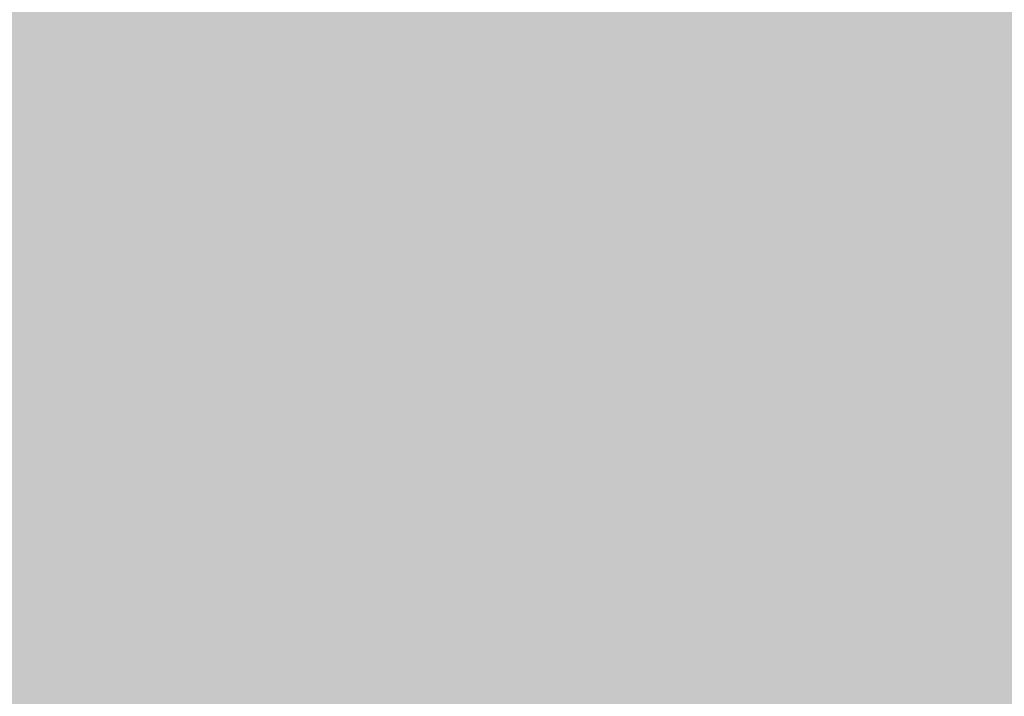
# Model space of a CAD drawing. Units: millimetres. Extents: x 0 to 2267, y 0 to 1823.
# Tile 75 of 256: x 1596.855 to 1600.369, y 1228.528 to 1230.942. Entities that reach past the tile are written whole.
import ezdxf

# ---------------------------------------------------------------- set-up
doc = ezdxf.new("R2010")
doc.units = ezdxf.units.MM
doc.header["$MEASUREMENT"] = 0
doc.layers.add('M-HATC', color=252, linetype='Continuous', lineweight=18)

msp = doc.modelspace()

# ---------------------------------------------------------------- hatches: boundary and pattern name
at = {"layer": 'M-HATC'}
h = msp.add_hatch(color=256, dxfattribs=at)
h.dxf.hatch_style = 1
h.paths.add_polyline_path([(2055.771, 1603.062), (1381.0868, 1603.062), (1381.0868, 1598.062), (2055.771, 1598.062)])
h.paths.add_polyline_path([(2055.771, 1598.062), (1381.0868, 1598.062), (1381.0868, 1593.062), (2055.771, 1593.062)])
h.paths.add_polyline_path([(2051.3074, 1536.7609), (1385.5504, 1536.7609), (1385.5504, 1526.7609), (1387.5504, 1526.7609), (1388.5366, 1525.0528), (1385.3319, 1521.2335), (1385.3319, 1521.2226), (2050.2542, 1522.7491), (2048.3212, 1525.0528), (2049.3074, 1526.7609), (2051.3074, 1526.7609)])
edge = h.paths.add_edge_path()
edge.add_arc((1847.5345, 1379.1492), 135, 222.603061, 222.890851, ccw=False)
edge.add_line((1748.1663, 1287.7656), (1683.0921, 1287.7656))
edge.add_arc((1583.7239, 1379.1492), 135, 317.109149, 317.396939, ccw=False)
edge.add_arc((1678.9686, 1290.6707), 5, 222.8909, 317.1091, ccw=False)
edge.add_arc((1774.2133, 1379.1492), 135, 222.603061, 222.890851, ccw=False)
edge.add_line((1674.8451, 1287.7656), (1609.7709, 1287.7656))
edge.add_arc((1510.4027, 1379.1492), 135, 317.109149, 317.396939, ccw=False)
edge.add_arc((1605.6474, 1290.6707), 5, 222.8909, 317.1091, ccw=False)
edge.add_arc((1700.8921, 1379.1492), 135, 222.603061, 222.890851, ccw=False)
edge.add_line((1601.5239, 1287.7656), (1536.4497, 1287.7656))
edge.add_arc((1437.0815, 1379.1492), 135, 317.109149, 317.396939, ccw=False)
edge.add_arc((1532.3262, 1290.6707), 5, 222.8909, 317.1091, ccw=False)
edge.add_arc((1627.5709, 1379.1492), 135, 222.603061, 222.890851, ccw=False)
edge.add_line((1528.2027, 1287.7656), (1505.9289, 1287.7656))
edge.add_spline(control_points=[(1505.9289, 1287.7656), (1504.2622, 1287.7656), (1504.2622, 1282.7656), (1505.9289, 1282.7656)], knot_values=[0, 0, 0, 0, 5, 5, 5, 5], degree=3, periodic=0)
edge.add_line((1505.9289, 1282.7656), (1930.9289, 1282.7656))
edge.add_spline(control_points=[(1930.9289, 1282.7656), (1932.5956, 1282.7656), (1932.5956, 1287.7656), (1930.9289, 1287.7656)], knot_values=[0, 0, 0, 0, 5, 5, 5, 5], degree=3, periodic=0)
edge.add_line((1930.9289, 1287.7656), (1903.0557, 1287.7656))
edge.add_arc((1803.6875, 1379.1492), 135, 317.109149, 317.396939, ccw=False)
edge.add_arc((1898.9322, 1290.6707), 5, 222.8909, 317.1091, ccw=False)
edge.add_arc((1994.1769, 1379.1492), 135, 222.603061, 222.890851, ccw=False)
edge.add_line((1894.8087, 1287.7656), (1829.7345, 1287.7656))
edge.add_arc((1730.3663, 1379.1492), 135, 317.109149, 317.396939, ccw=False)
edge.add_arc((1825.611, 1290.6707), 5, 222.8909, 317.1091, ccw=False)
edge.add_arc((1920.8557, 1379.1492), 135, 222.603061, 222.890851, ccw=False)
edge.add_line((1821.4875, 1287.7656), (1756.4133, 1287.7656))
edge.add_arc((1657.0451, 1379.1492), 135, 317.109149, 317.396939, ccw=False)
edge.add_arc((1752.2898, 1290.6707), 5, 222.8909, 317.1091, ccw=False)
edge = h.paths.add_edge_path()
edge.add_spline(control_points=[(1843.4289, 1227.2475), (1845.0956, 1227.2475), (1845.0956, 1232.2475), (1843.4289, 1232.2475)], knot_values=[0, 0, 0, 0, 5, 5, 5, 5], degree=3, periodic=0)
edge.add_line((1843.4289, 1232.2475), (1593.4289, 1232.2475))
edge.add_spline(control_points=[(1593.4289, 1232.2475), (1591.7622, 1232.2475), (1591.7622, 1227.2475), (1593.4289, 1227.2475)], knot_values=[0, 0, 0, 0, 5, 5, 5, 5], degree=3, periodic=0)
edge.add_line((1593.4289, 1227.2475), (1843.4289, 1227.2475))
h.paths.add_polyline_path([(1905.9289, 1127.4171), (1530.9289, 1127.4171, 0.414214), (1520.9289, 1117.4171), (1530.9289, 1117.4171), (1915.9289, 1117.4171, 0.414214)])
edge = h.paths.add_edge_path()
edge.add_arc((1397.0858, 1498.4078), 12.7299, 90.78215, 190.87871, ccw=False)
edge.add_line((1396.912, 1511.1365), (1428.0097, 1511.3488))
edge.add_line((1428.0097, 1511.3488), (1433.0097, 1511.3488))
edge.add_line((1433.0097, 1511.3488), (1434.439, 1511.3488))
edge.add_arc((1419.474, 1498.0804), 20, 41.561, 74.08211)
edge.add_line((1424.9592, 1517.3135), (1399.9351, 1517.2561))
edge.add_spline(control_points=[(1399.9307, 1517.2561), (1399.884, 1517.2131), (1399.8328, 1517.1689), (1399.7774, 1517.1236)], knot_values=[11.567499, 11.567499, 11.567499, 11.567499, 11.814249, 11.814249, 11.814249, 11.814249], degree=3, periodic=0)
edge.add_spline(control_points=[(1399.6328, 1517.0099), (1399.5831, 1516.9721), (1399.5307, 1516.9338), (1399.4759, 1516.8947)], knot_values=[11.167718, 11.167718, 11.167718, 11.167718, 11.365188, 11.365188, 11.365188, 11.365188], degree=3, periodic=0)
edge.add_spline(control_points=[(1399.3398, 1516.8001), (1399.1514, 1516.6719), (1398.9384, 1516.5377), (1398.704, 1516.3994)], knot_values=[10.376405, 10.376405, 10.376405, 10.376405, 11.00994, 11.00994, 11.00994, 11.00994], degree=3, periodic=0)
edge.add_spline(control_points=[(1398.6572, 1516.3719), (1398.5789, 1516.326), (1398.4983, 1516.2797), (1398.4155, 1516.2331)], knot_values=[10.125175, 10.125175, 10.125175, 10.125175, 10.334406, 10.334406, 10.334406, 10.334406], degree=3, periodic=0)
edge.add_spline(control_points=[(1398.2642, 1516.1487), (1398.196, 1516.1111), (1398.1263, 1516.0732), (1398.0555, 1516.0351)], knot_values=[9.832246, 9.832246, 9.832246, 9.832246, 9.999658, 9.999658, 9.999658, 9.999658], degree=3, periodic=0)
edge.add_spline(control_points=[(1397.9987, 1516.0048), (1397.7312, 1515.8621), (1397.446, 1515.7171), (1397.1466, 1515.5714)], knot_values=[9.161808, 9.161808, 9.161808, 9.161808, 9.787769, 9.787769, 9.787769, 9.787769], degree=3, periodic=0)
edge.add_spline(control_points=[(1397.1466, 1515.5714), (1396.8418, 1515.423), (1396.5222, 1515.274), (1396.1914, 1515.1262)], knot_values=[8.524455, 8.524455, 8.524455, 8.524455, 9.161808, 9.161808, 9.161808, 9.161808], degree=3, periodic=0)
edge.add_spline(control_points=[(1396.0777, 1515.0756), (1395.9854, 1515.0348), (1395.8922, 1514.994), (1395.7983, 1514.9534)], knot_values=[8.275193, 8.275193, 8.275193, 8.275193, 8.451726, 8.451726, 8.451726, 8.451726], degree=3, periodic=0)
edge.add_spline(control_points=[(1395.6018, 1514.8691), (1395.4997, 1514.8257), (1395.3968, 1514.7824), (1395.2932, 1514.7394)], knot_values=[7.962917, 7.962917, 7.962917, 7.962917, 8.152764, 8.152764, 8.152764, 8.152764], degree=3, periodic=0)
edge.add_spline(control_points=[(1395.2116, 1514.7057), (1394.8278, 1514.5475), (1394.4345, 1514.3929), (1394.0364, 1514.2442)], knot_values=[7.21254, 7.21254, 7.21254, 7.21254, 7.913148, 7.913148, 7.913148, 7.913148], degree=3, periodic=0)
edge.add_spline(control_points=[(1394.0364, 1514.2442), (1393.7076, 1514.1214), (1393.3754, 1514.0027), (1393.0427, 1513.8895)], knot_values=[6.633733, 6.633733, 6.633733, 6.633733, 7.21254, 7.21254, 7.21254, 7.21254], degree=3, periodic=0)
edge.add_spline(control_points=[(1392.8214, 1513.815), (1392.7198, 1513.7812), (1392.6181, 1513.7479), (1392.5166, 1513.7152)], knot_values=[6.328796, 6.328796, 6.328796, 6.328796, 6.505493, 6.505493, 6.505493, 6.505493], degree=3, periodic=0)
edge.add_spline(control_points=[(1392.5166, 1513.7152), (1392.3187, 1513.6515), (1392.1212, 1513.59), (1391.9244, 1513.531)], knot_values=[5.984605, 5.984605, 5.984605, 5.984605, 6.328796, 6.328796, 6.328796, 6.328796], degree=3, periodic=0)
edge.add_spline(control_points=[(1391.7915, 1513.4915), (1391.3122, 1513.3501), (1390.8384, 1513.2239), (1390.3784, 1513.1171)], knot_values=[5.066697, 5.066697, 5.066697, 5.066697, 5.907055, 5.907055, 5.907055, 5.907055], degree=3, periodic=0)
edge.add_spline(control_points=[(1390.3784, 1513.1171), (1390.1797, 1513.071), (1389.9836, 1513.0284), (1389.7907, 1512.9899)], knot_values=[4.70367, 4.70367, 4.70367, 4.70367, 5.066695, 5.066695, 5.066695, 5.066695], degree=3, periodic=0)
edge.add_spline(control_points=[(1389.422, 1512.9204), (1389.2459, 1512.8892), (1389.0729, 1512.8617), (1388.9036, 1512.8381)], knot_values=[4.130571, 4.130571, 4.130571, 4.130571, 4.469816, 4.469816, 4.469816, 4.469816], degree=3, periodic=0)
edge.add_spline(control_points=[(1388.9036, 1512.8381), (1388.591, 1512.7946), (1388.2911, 1512.7644), (1388.0071, 1512.7494)], knot_values=[3.504031, 3.504031, 3.504031, 3.504031, 4.130571, 4.130571, 4.130571, 4.130571], degree=3, periodic=0)
edge.add_spline(control_points=[(1387.9356, 1512.7459), (1387.8538, 1512.7423), (1387.7733, 1512.74), (1387.6944, 1512.739)], knot_values=[3.268866, 3.268866, 3.268866, 3.268866, 3.451164, 3.451164, 3.451164, 3.451164], degree=3, periodic=0)
edge.add_spline(control_points=[(1387.3351, 1512.7443), (1387.2076, 1512.7499), (1387.0847, 1512.7597), (1386.967, 1512.7739)], knot_values=[2.670686, 2.670686, 2.670686, 2.670686, 2.984, 2.984, 2.984, 2.984], degree=3, periodic=0)
edge.add_spline(control_points=[(1386.8327, 1512.7922), (1386.8209, 1512.7941), (1386.8092, 1512.7959), (1386.7975, 1512.7979)], knot_values=[2.516981, 2.516981, 2.516981, 2.516981, 2.549528, 2.549528, 2.549528, 2.549528], degree=3, periodic=0)
edge.add_spline(control_points=[(1386.4526, 1512.8735), (1386.4257, 1512.881), (1386.3993, 1512.889), (1386.3733, 1512.8972)], knot_values=[2.095869, 2.095869, 2.095869, 2.095869, 2.17941, 2.17941, 2.17941, 2.17941], degree=3, periodic=0)
edge.add_spline(control_points=[(1386.0691, 1513.0189), (1386.0634, 1513.0217), (1386.0577, 1513.0246), (1386.052, 1513.0275)], knot_values=[1.72453, 1.72453, 1.72453, 1.72453, 1.745933, 1.745933, 1.745933, 1.745933], degree=3, periodic=0)
edge.add_arc((1399.474, 1498.0804), 20, 131.82432, 180)
edge.add_arc((1630.3336, 1505.5484), 250.9708, 181.705176, 236.427975)
edge.add_arc((1605.3399, 1483.3044), 218.7822, 238.660829, 243.34961)
edge.add_arc((1647.0911, 1510.3592), 262.8986, 183.129836, 237.853442, ccw=False)
h.paths.add_polyline_path([(1406.5369, 1391.9644, 0.149382), (1491.5506, 1296.4418, -0.129517)], flags=17)
edge = h.paths.add_edge_path()
edge.add_arc((2037.3838, 1498.0804), 20, 0, 48.26587)
edge.add_spline(control_points=[(2050.6973, 1513.0052), (2050.6512, 1512.9847), (2050.6034, 1512.9655), (2050.5539, 1512.9477)], knot_values=[1.835652, 1.835652, 1.835652, 1.835652, 2.000781, 2.000781, 2.000781, 2.000781], degree=3, periodic=0)
edge.add_spline(control_points=[(2050.4616, 1512.9166), (2050.479, 1512.9221), (2050.4963, 1512.9277), (2050.5133, 1512.9335)], knot_values=[2.045477, 2.045477, 2.045477, 2.045477, 2.101389, 2.101389, 2.101389, 2.101389], degree=3, periodic=0)
edge.add_spline(control_points=[(2050.129, 1512.8342), (2050.1984, 1512.8473), (2050.2657, 1512.8623), (2050.3308, 1512.8792)], knot_values=[2.237629, 2.237629, 2.237629, 2.237629, 2.435841, 2.435841, 2.435841, 2.435841], degree=3, periodic=0)
edge.add_spline(control_points=[(2050.0946, 1512.8278), (2050.1061, 1512.8299), (2050.1176, 1512.832), (2050.129, 1512.8342)], knot_values=[2.435841, 2.435841, 2.435841, 2.435841, 2.468321, 2.468321, 2.468321, 2.468321], degree=3, periodic=0)
edge.add_spline(control_points=[(2049.7843, 1512.7851), (2049.8552, 1512.7922), (2049.9243, 1512.8008), (2049.9917, 1512.8109)], knot_values=[2.563852, 2.563852, 2.563852, 2.563852, 2.748541, 2.748541, 2.748541, 2.748541], degree=3, periodic=0)
edge.add_spline(control_points=[(2049.4052, 1512.7617), (2049.5364, 1512.7653), (2049.6629, 1512.773), (2049.7843, 1512.7851)], knot_values=[2.748541, 2.748541, 2.748541, 2.748541, 3.064882, 3.064882, 3.064882, 3.064882], degree=3, periodic=0)
edge.add_spline(control_points=[(2049.1698, 1512.7597), (2049.2336, 1512.7591), (2049.2965, 1512.7594), (2049.3584, 1512.7606)], knot_values=[3.102309, 3.102309, 3.102309, 3.102309, 3.2503, 3.2503, 3.2503, 3.2503], degree=3, periodic=0)
edge.add_spline(control_points=[(2048.8573, 1512.7691), (2048.9638, 1512.7638), (2049.068, 1512.7606), (2049.1698, 1512.7597)], knot_values=[3.2503, 3.2503, 3.2503, 3.2503, 3.486069, 3.486069, 3.486069, 3.486069], degree=3, periodic=0)
edge.add_spline(control_points=[(2048.6924, 1512.7789), (2048.3729, 1512.8009), (2048.0345, 1512.8411), (2047.6817, 1512.897)], knot_values=[3.606429, 3.606429, 3.606429, 3.606429, 4.2989, 4.2989, 4.2989, 4.2989], degree=3, periodic=0)
edge.add_spline(control_points=[(2047.6817, 1512.897), (2047.5458, 1512.9185), (2047.4077, 1512.9424), (2047.2678, 1512.9685)], knot_values=[4.2989, 4.2989, 4.2989, 4.2989, 4.565769, 4.565769, 4.565769, 4.565769], degree=3, periodic=0)
edge.add_spline(control_points=[(2047.2678, 1512.9685), (2047.1449, 1512.9914), (2047.0207, 1513.016), (2046.8951, 1513.0422)], knot_values=[4.565769, 4.565769, 4.565769, 4.565769, 4.799971, 4.799971, 4.799971, 4.799971], degree=3, periodic=0)
edge.add_spline(control_points=[(2046.8951, 1513.0422), (2046.5286, 1513.1188), (2046.1513, 1513.209), (2045.7676, 1513.3107)], knot_values=[4.799971, 4.799971, 4.799971, 4.799971, 5.483718, 5.483718, 5.483718, 5.483718], degree=3, periodic=0)
edge.add_spline(control_points=[(2045.7676, 1513.3107), (2045.3724, 1513.4154), (2044.9704, 1513.5322), (2044.5662, 1513.6588)], knot_values=[5.483718, 5.483718, 5.483718, 5.483718, 6.187866, 6.187866, 6.187866, 6.187866], degree=3, periodic=0)
edge.add_spline(control_points=[(2044.5662, 1513.6588), (2044.4149, 1513.7061), (2044.2633, 1513.7549), (2044.1116, 1513.8048)], knot_values=[6.187866, 6.187866, 6.187866, 6.187866, 6.451551, 6.451551, 6.451551, 6.451551], degree=3, periodic=0)
edge.add_spline(control_points=[(2044.1116, 1513.8048), (2043.9967, 1513.8427), (2043.8817, 1513.8813), (2043.7668, 1513.9205)], knot_values=[6.451551, 6.451551, 6.451551, 6.451551, 6.651434, 6.651434, 6.651434, 6.651434], degree=3, periodic=0)
edge.add_spline(control_points=[(2043.7668, 1513.9205), (2043.3716, 1514.0554), (2042.9774, 1514.1979), (2042.5886, 1514.3458)], knot_values=[6.651434, 6.651434, 6.651434, 6.651434, 7.338879, 7.338879, 7.338879, 7.338879], degree=3, periodic=0)
edge.add_spline(control_points=[(2042.5886, 1514.3458), (2042.1643, 1514.5071), (2041.7465, 1514.6749), (2041.3409, 1514.846)], knot_values=[7.338879, 7.338879, 7.338879, 7.338879, 8.089209, 8.089209, 8.089209, 8.089209], degree=3, periodic=0)
edge.add_spline(control_points=[(2041.3409, 1514.846), (2041.1028, 1514.9465), (2040.869, 1515.0481), (2040.6405, 1515.1502)], knot_values=[8.089209, 8.089209, 8.089209, 8.089209, 8.529587, 8.529587, 8.529587, 8.529587], degree=3, periodic=0)
edge.add_spline(control_points=[(2040.51, 1515.2089), (2040.0824, 1515.4022), (2039.6747, 1515.5971), (2039.295, 1515.7894)], knot_values=[8.613818, 8.613818, 8.613818, 8.613818, 9.44571, 9.44571, 9.44571, 9.44571], degree=3, periodic=0)
edge.add_spline(control_points=[(2039.295, 1515.7894), (2039.0618, 1515.9075), (2038.8391, 1516.0246), (2038.6288, 1516.1398)], knot_values=[9.44571, 9.44571, 9.44571, 9.44571, 9.956404, 9.956404, 9.956404, 9.956404], degree=3, periodic=0)
edge.add_spline(control_points=[(2038.6288, 1516.1398), (2038.5187, 1516.2001), (2038.4121, 1516.2598), (2038.309, 1516.3189)], knot_values=[9.956404, 9.956404, 9.956404, 9.956404, 10.223542, 10.223542, 10.223542, 10.223542], degree=3, periodic=0)
edge.add_spline(control_points=[(2038.309, 1516.3189), (2038.2138, 1516.3735), (2038.1216, 1516.4276), (2038.0328, 1516.481)], knot_values=[10.223542, 10.223542, 10.223542, 10.223542, 10.47051, 10.47051, 10.47051, 10.47051], degree=3, periodic=0)
edge.add_spline(control_points=[(2038.0328, 1516.481), (2037.7855, 1516.6296), (2037.5639, 1516.773), (2037.3722, 1516.909)], knot_values=[10.47051, 10.47051, 10.47051, 10.47051, 11.15767, 11.15767, 11.15767, 11.15767], degree=3, periodic=0)
edge.add_spline(control_points=[(2037.3722, 1516.909), (2037.2789, 1516.9752), (2037.1927, 1517.0396), (2037.1142, 1517.102)], knot_values=[11.15767, 11.15767, 11.15767, 11.15767, 11.49227, 11.49227, 11.49227, 11.49227], degree=3, periodic=0)
edge.add_spline(control_points=[(2036.8564, 1517.3259), (2036.9148, 1517.2692), (2036.9814, 1517.2103), (2037.0557, 1517.1492)], knot_values=[11.577341, 11.577341, 11.577341, 11.577341, 11.91035, 11.91035, 11.91035, 11.91035], degree=3, periodic=0)
edge.add_spline(control_points=[(2036.8074, 1517.3748), (2036.823, 1517.3587), (2036.8393, 1517.3424), (2036.8564, 1517.3259)], knot_values=[11.91035, 11.91035, 11.91035, 11.91035, 12.007402, 12.007402, 12.007402, 12.007402], degree=3, periodic=0)
edge.add_spline(control_points=[(2036.7017, 1517.494), (2036.7104, 1517.483), (2036.7196, 1517.4719), (2036.7291, 1517.4606)], knot_values=[12.184155, 12.184155, 12.184155, 12.184155, 12.255409, 12.255409, 12.255409, 12.255409], degree=3, periodic=0)
edge.add_spline(control_points=[(2036.6159, 1517.6205), (2036.62, 1517.613), (2036.6243, 1517.6055), (2036.6289, 1517.5979)], knot_values=[12.487913, 12.487913, 12.487913, 12.487913, 12.541035, 12.541035, 12.541035, 12.541035], degree=3, periodic=0)
edge.add_spline(control_points=[(2036.5635, 1517.786), (2036.5637, 1517.7794), (2036.5642, 1517.7726), (2036.565, 1517.7658)], knot_values=[12.911761, 12.911761, 12.911761, 12.911761, 12.968286, 12.968286, 12.968286, 12.968286], degree=3, periodic=0)
edge.add_spline(control_points=[(2036.6166, 1517.9304), (2036.6125, 1517.9259), (2036.6086, 1517.9212), (2036.6049, 1517.9165)], knot_values=[13.382527, 13.382527, 13.382527, 13.382527, 13.433791, 13.433791, 13.433791, 13.433791], degree=3, periodic=0)
edge.add_spline(control_points=[(2036.749, 1518.017), (2036.7361, 1518.0116), (2036.7239, 1518.006), (2036.7124, 1518.0002)], knot_values=[13.726299, 13.726299, 13.726299, 13.726299, 13.809928, 13.809928, 13.809928, 13.809928], degree=3, periodic=0)
edge.add_spline(control_points=[(2036.8604, 1518.0528), (2036.8386, 1518.0474), (2036.8181, 1518.0416), (2036.7988, 1518.0353)], knot_values=[13.910887, 13.910887, 13.910887, 13.910887, 14.02153, 14.02153, 14.02153, 14.02153], degree=3, periodic=0)
edge.add_line((2036.9639, 1518.0804), (2032.3838, 1518.0804))
edge.add_line((2032.3838, 1518.0804), (2027.3838, 1518.0804))
edge.add_line((2027.3838, 1518.0804), (2022.3838, 1518.0804))
edge.add_line((2022.3838, 1518.0804), (2017.3838, 1518.0804))
edge.add_arc((2017.3838, 1498.0804), 20, 90, 138.439)
edge.add_line((2002.4188, 1511.3488), (2003.8481, 1511.3488))
edge.add_line((2003.8481, 1511.3488), (2008.8481, 1511.3488))
edge.add_line((2008.8481, 1511.3488), (2039.772, 1511.1377))
edge.add_arc((2039.772, 1498.4078), 12.7299, -10.87871, 90, ccw=False)
edge.add_arc((1789.7668, 1510.3592), 262.8986, 302.146558, 356.870164, ccw=False)
edge.add_arc((1831.5179, 1483.3044), 218.7822, 296.65039, 301.339171)
edge.add_arc((1806.5242, 1505.5484), 250.9708, 303.572025, 358.294824)
h.paths.add_polyline_path([(2030.321, 1391.9644, -0.129517), (1945.3072, 1296.4418, 0.149382)], flags=17)
edge = h.paths.add_edge_path()
edge.add_spline(control_points=[(2037.2464, 1518.0821), (2037.2898, 1518.081), (2037.3355, 1518.0804), (2037.3838, 1518.0804)], knot_values=[0.000012, 0.000012, 0.000012, 0.000012, 0.144754, 0.144754, 0.144754, 0.144754], degree=3, periodic=0)
edge.add_line((2037.3357, 1518.0804), (2037.0096, 1518.0804))
edge.add_spline(control_points=[(2037.0096, 1518.0804), (2036.9822, 1518.0768), (2036.956, 1518.0727), (2036.9312, 1518.0681)], knot_values=[14.13465, 14.13465, 14.13465, 14.13465, 14.247197, 14.247197, 14.247197, 14.247197], degree=3, periodic=0)
edge.add_spline(control_points=[(2036.9312, 1518.0681), (2036.9276, 1518.0674), (2036.9241, 1518.0667), (2036.9205, 1518.0661)], knot_values=[14.118315, 14.118315, 14.118315, 14.118315, 14.13465, 14.13465, 14.13465, 14.13465], degree=3, periodic=0)
edge.add_spline(control_points=[(2036.9205, 1518.0661), (2036.9118, 1518.0644), (2036.9032, 1518.0626), (2036.8948, 1518.0608)], knot_values=[14.078086, 14.078086, 14.078086, 14.078086, 14.118315, 14.118315, 14.118315, 14.118315], degree=3, periodic=0)
edge.add_spline(control_points=[(2036.8948, 1518.0608), (2036.883, 1518.0583), (2036.8716, 1518.0556), (2036.8604, 1518.0528)], knot_values=[14.02153, 14.02153, 14.02153, 14.02153, 14.078086, 14.078086, 14.078086, 14.078086], degree=3, periodic=0)
edge.add_spline(control_points=[(2036.8604, 1518.0528), (2036.8386, 1518.0474), (2036.8181, 1518.0416), (2036.7988, 1518.0353)], knot_values=[13.910887, 13.910887, 13.910887, 13.910887, 14.02153, 14.02153, 14.02153, 14.02153], degree=3, periodic=0)
edge.add_spline(control_points=[(2036.7988, 1518.0353), (2036.7981, 1518.035), (2036.7974, 1518.0348), (2036.7967, 1518.0346)], knot_values=[13.906906, 13.906906, 13.906906, 13.906906, 13.910887, 13.910887, 13.910887, 13.910887], degree=3, periodic=0)
edge.add_spline(control_points=[(2036.7967, 1518.0346), (2036.7882, 1518.0318), (2036.7799, 1518.0289), (2036.7719, 1518.0259)], knot_values=[13.857826, 13.857826, 13.857826, 13.857826, 13.906906, 13.906906, 13.906906, 13.906906], degree=3, periodic=0)
edge.add_spline(control_points=[(2036.7719, 1518.0259), (2036.764, 1518.023), (2036.7564, 1518.02), (2036.749, 1518.017)], knot_values=[13.809928, 13.809928, 13.809928, 13.809928, 13.857826, 13.857826, 13.857826, 13.857826], degree=3, periodic=0)
edge.add_spline(control_points=[(2036.749, 1518.017), (2036.7361, 1518.0116), (2036.7239, 1518.006), (2036.7124, 1518.0002)], knot_values=[13.726299, 13.726299, 13.726299, 13.726299, 13.809928, 13.809928, 13.809928, 13.809928], degree=3, periodic=0)
edge.add_spline(control_points=[(2036.7124, 1518.0002), (2036.7121, 1518), (2036.7118, 1517.9999), (2036.7115, 1517.9997)], knot_values=[13.723993, 13.723993, 13.723993, 13.723993, 13.726299, 13.726299, 13.726299, 13.726299], degree=3, periodic=0)
edge.add_spline(control_points=[(2036.7115, 1517.9997), (2036.7063, 1517.9971), (2036.7013, 1517.9944), (2036.6965, 1517.9917)], knot_values=[13.686536, 13.686536, 13.686536, 13.686536, 13.723993, 13.723993, 13.723993, 13.723993], degree=3, periodic=0)
edge.add_spline(control_points=[(2036.6965, 1517.9917), (2036.6919, 1517.9891), (2036.6874, 1517.9865), (2036.6831, 1517.9839)], knot_values=[13.651251, 13.651251, 13.651251, 13.651251, 13.686536, 13.686536, 13.686536, 13.686536], degree=3, periodic=0)
edge.add_spline(control_points=[(2036.6831, 1517.9839), (2036.6764, 1517.9798), (2036.67, 1517.9757), (2036.6639, 1517.9714)], knot_values=[13.596804, 13.596804, 13.596804, 13.596804, 13.651251, 13.651251, 13.651251, 13.651251], degree=3, periodic=0)
edge.add_spline(control_points=[(2036.6639, 1517.9714), (2036.6636, 1517.9712), (2036.6633, 1517.9709), (2036.6629, 1517.9707)], knot_values=[13.593956, 13.593956, 13.593956, 13.593956, 13.596804, 13.596804, 13.596804, 13.596804], degree=3, periodic=0)
edge.add_spline(control_points=[(2036.6629, 1517.9707), (2036.6603, 1517.9689), (2036.6577, 1517.967), (2036.6552, 1517.9651)], knot_values=[13.570322, 13.570322, 13.570322, 13.570322, 13.593956, 13.593956, 13.593956, 13.593956], degree=3, periodic=0)
edge.add_spline(control_points=[(2036.6552, 1517.9651), (2036.6525, 1517.9631), (2036.6499, 1517.9611), (2036.6474, 1517.9591)], knot_values=[13.545477, 13.545477, 13.545477, 13.545477, 13.570322, 13.570322, 13.570322, 13.570322], degree=3, periodic=0)
edge.add_spline(control_points=[(2036.6474, 1517.9591), (2036.6472, 1517.9589), (2036.6471, 1517.9588), (2036.6469, 1517.9587)], knot_values=[13.543931, 13.543931, 13.543931, 13.543931, 13.545477, 13.545477, 13.545477, 13.545477], degree=3, periodic=0)
edge.add_spline(control_points=[(2036.6469, 1517.9587), (2036.6412, 1517.9541), (2036.6358, 1517.9494), (2036.6307, 1517.9447)], knot_values=[13.488237, 13.488237, 13.488237, 13.488237, 13.543931, 13.543931, 13.543931, 13.543931], degree=3, periodic=0)
edge.add_spline(control_points=[(2036.6307, 1517.9447), (2036.6282, 1517.9423), (2036.6257, 1517.9399), (2036.6233, 1517.9374)], knot_values=[13.460307, 13.460307, 13.460307, 13.460307, 13.488237, 13.488237, 13.488237, 13.488237], degree=3, periodic=0)
edge.add_spline(control_points=[(2036.6233, 1517.9374), (2036.6215, 1517.9356), (2036.6198, 1517.9338), (2036.6181, 1517.932)], knot_values=[13.439712, 13.439712, 13.439712, 13.439712, 13.460307, 13.460307, 13.460307, 13.460307], degree=3, periodic=0)
edge.add_spline(control_points=[(2036.6181, 1517.932), (2036.6176, 1517.9315), (2036.6171, 1517.9309), (2036.6166, 1517.9304)], knot_values=[13.433791, 13.433791, 13.433791, 13.433791, 13.439712, 13.439712, 13.439712, 13.439712], degree=3, periodic=0)
edge.add_spline(control_points=[(2036.6166, 1517.9304), (2036.6125, 1517.9259), (2036.6086, 1517.9212), (2036.6049, 1517.9165)], knot_values=[13.382527, 13.382527, 13.382527, 13.382527, 13.433791, 13.433791, 13.433791, 13.433791], degree=3, periodic=0)
edge.add_spline(control_points=[(2036.6049, 1517.9165), (2036.6026, 1517.9135), (2036.6004, 1517.9104), (2036.5982, 1517.9074)], knot_values=[13.350017, 13.350017, 13.350017, 13.350017, 13.382527, 13.382527, 13.382527, 13.382527], degree=3, periodic=0)
edge.add_spline(control_points=[(2036.5982, 1517.9074), (2036.5972, 1517.9059), (2036.5962, 1517.9043), (2036.5952, 1517.9028)], knot_values=[13.333922, 13.333922, 13.333922, 13.333922, 13.350017, 13.350017, 13.350017, 13.350017], degree=3, periodic=0)
edge.add_spline(control_points=[(2036.5952, 1517.9028), (2036.5945, 1517.9018), (2036.5939, 1517.9009), (2036.5933, 1517.8999)], knot_values=[13.323828, 13.323828, 13.323828, 13.323828, 13.333922, 13.333922, 13.333922, 13.333922], degree=3, periodic=0)
edge.add_spline(control_points=[(2036.5933, 1517.8999), (2036.5905, 1517.8955), (2036.5879, 1517.8909), (2036.5855, 1517.8864)], knot_values=[13.277545, 13.277545, 13.277545, 13.277545, 13.323828, 13.323828, 13.323828, 13.323828], degree=3, periodic=0)
edge.add_spline(control_points=[(2036.5855, 1517.8864), (2036.5836, 1517.8827), (2036.5817, 1517.8789), (2036.5801, 1517.8751)], knot_values=[13.240119, 13.240119, 13.240119, 13.240119, 13.277545, 13.277545, 13.277545, 13.277545], degree=3, periodic=0)
edge.add_spline(control_points=[(2036.5801, 1517.8751), (2036.5795, 1517.8739), (2036.579, 1517.8727), (2036.5785, 1517.8715)], knot_values=[13.228211, 13.228211, 13.228211, 13.228211, 13.240119, 13.240119, 13.240119, 13.240119], degree=3, periodic=0)
edge.add_spline(control_points=[(2036.5785, 1517.8715), (2036.578, 1517.8702), (2036.5774, 1517.869), (2036.5769, 1517.8677)], knot_values=[13.215717, 13.215717, 13.215717, 13.215717, 13.228211, 13.228211, 13.228211, 13.228211], degree=3, periodic=0)
edge.add_spline(control_points=[(2036.5769, 1517.8677), (2036.5755, 1517.864), (2036.5741, 1517.8603), (2036.5729, 1517.8565)], knot_values=[13.179847, 13.179847, 13.179847, 13.179847, 13.215717, 13.215717, 13.215717, 13.215717], degree=3, periodic=0)
edge.add_spline(control_points=[(2036.5729, 1517.8565), (2036.5713, 1517.8515), (2036.5699, 1517.8464), (2036.5687, 1517.8413)], knot_values=[13.132017, 13.132017, 13.132017, 13.132017, 13.179847, 13.179847, 13.179847, 13.179847], degree=3, periodic=0)
edge.add_spline(control_points=[(2036.5687, 1517.8413), (2036.5684, 1517.8402), (2036.5682, 1517.8392), (2036.568, 1517.8382)], knot_values=[13.122482, 13.122482, 13.122482, 13.122482, 13.132017, 13.132017, 13.132017, 13.132017], degree=3, periodic=0)
edge.add_spline(control_points=[(2036.568, 1517.8382), (2036.5676, 1517.8363), (2036.5672, 1517.8345), (2036.5669, 1517.8327)], knot_values=[13.105592, 13.105592, 13.105592, 13.105592, 13.122482, 13.122482, 13.122482, 13.122482], degree=3, periodic=0)
edge.add_spline(control_points=[(2036.5669, 1517.8327), (2036.5662, 1517.8292), (2036.5657, 1517.8257), (2036.5652, 1517.8222)], knot_values=[13.074063, 13.074063, 13.074063, 13.074063, 13.105592, 13.105592, 13.105592, 13.105592], degree=3, periodic=0)
edge.add_spline(control_points=[(2036.5652, 1517.8222), (2036.5652, 1517.8222), (2036.5652, 1517.8222), (2036.5652, 1517.8222)], knot_values=[13.074043, 13.074043, 13.074043, 13.074043, 13.074063, 13.074063, 13.074063, 13.074063], degree=3, periodic=0)
edge.add_spline(control_points=[(2036.5652, 1517.8222), (2036.5644, 1517.8164), (2036.5639, 1517.8106), (2036.5636, 1517.8046)], knot_values=[13.021884, 13.021884, 13.021884, 13.021884, 13.074043, 13.074043, 13.074043, 13.074043], degree=3, periodic=0)
edge.add_spline(control_points=[(2036.5636, 1517.8046), (2036.5636, 1517.804), (2036.5636, 1517.8034), (2036.5635, 1517.8028)], knot_values=[13.01674, 13.01674, 13.01674, 13.01674, 13.021884, 13.021884, 13.021884, 13.021884], degree=3, periodic=0)
edge.add_spline(control_points=[(2036.5635, 1517.8028), (2036.5634, 1517.8005), (2036.5634, 1517.7982), (2036.5634, 1517.7958)], knot_values=[12.996438, 12.996438, 12.996438, 12.996438, 13.01674, 13.01674, 13.01674, 13.01674], degree=3, periodic=0)
edge.add_spline(control_points=[(2036.5634, 1517.7958), (2036.5633, 1517.7926), (2036.5634, 1517.7893), (2036.5635, 1517.786)], knot_values=[12.968286, 12.968286, 12.968286, 12.968286, 12.996438, 12.996438, 12.996438, 12.996438], degree=3, periodic=0)
edge.add_spline(control_points=[(2036.5635, 1517.786), (2036.5637, 1517.7794), (2036.5642, 1517.7726), (2036.565, 1517.7658)], knot_values=[12.911761, 12.911761, 12.911761, 12.911761, 12.968286, 12.968286, 12.968286, 12.968286], degree=3, periodic=0)
edge.add_spline(control_points=[(2036.565, 1517.7658), (2036.565, 1517.7657), (2036.565, 1517.7656), (2036.565, 1517.7656)], knot_values=[12.911017, 12.911017, 12.911017, 12.911017, 12.911761, 12.911761, 12.911761, 12.911761], degree=3, periodic=0)
edge.add_spline(control_points=[(2036.565, 1517.7656), (2036.5654, 1517.7625), (2036.5658, 1517.7593), (2036.5663, 1517.7562)], knot_values=[12.88528, 12.88528, 12.88528, 12.88528, 12.911017, 12.911017, 12.911017, 12.911017], degree=3, periodic=0)
edge.add_spline(control_points=[(2036.5663, 1517.7562), (2036.5667, 1517.7534), (2036.5672, 1517.7506), (2036.5677, 1517.7478)], knot_values=[12.862519, 12.862519, 12.862519, 12.862519, 12.88528, 12.88528, 12.88528, 12.88528], degree=3, periodic=0)
edge.add_spline(control_points=[(2036.5677, 1517.7478), (2036.5678, 1517.7474), (2036.5679, 1517.7469), (2036.568, 1517.7465)], knot_values=[12.858885, 12.858885, 12.858885, 12.858885, 12.862519, 12.862519, 12.862519, 12.862519], degree=3, periodic=0)
edge.add_spline(control_points=[(2036.568, 1517.7465), (2036.5692, 1517.7399), (2036.5707, 1517.7332), (2036.5724, 1517.7264)], knot_values=[12.8053, 12.8053, 12.8053, 12.8053, 12.858885, 12.858885, 12.858885, 12.858885], degree=3, periodic=0)
edge.add_spline(control_points=[(2036.5724, 1517.7264), (2036.5734, 1517.7226), (2036.5745, 1517.7187), (2036.5756, 1517.7149)], knot_values=[12.775176, 12.775176, 12.775176, 12.775176, 12.8053, 12.8053, 12.8053, 12.8053], degree=3, periodic=0)
edge.add_spline(control_points=[(2036.5756, 1517.7149), (2036.5763, 1517.7125), (2036.577, 1517.7102), (2036.5778, 1517.7078)], knot_values=[12.756759, 12.756759, 12.756759, 12.756759, 12.775176, 12.775176, 12.775176, 12.775176], degree=3, periodic=0)
edge.add_spline(control_points=[(2036.5778, 1517.7078), (2036.5781, 1517.7067), (2036.5784, 1517.7057), (2036.5787, 1517.7047)], knot_values=[12.748742, 12.748742, 12.748742, 12.748742, 12.756759, 12.756759, 12.756759, 12.756759], degree=3, periodic=0)
edge.add_spline(control_points=[(2036.5787, 1517.7047), (2036.5808, 1517.6983), (2036.5831, 1517.6919), (2036.5856, 1517.6854)], knot_values=[12.69959, 12.69959, 12.69959, 12.69959, 12.748742, 12.748742, 12.748742, 12.748742], degree=3, periodic=0)
edge.add_spline(control_points=[(2036.5856, 1517.6854), (2036.5876, 1517.68), (2036.5898, 1517.6746), (2036.5921, 1517.6692)], knot_values=[12.659038, 12.659038, 12.659038, 12.659038, 12.69959, 12.69959, 12.69959, 12.69959], degree=3, periodic=0)
edge.add_spline(control_points=[(2036.5921, 1517.6692), (2036.594, 1517.6648), (2036.5959, 1517.6605), (2036.5979, 1517.6561)], knot_values=[12.626806, 12.626806, 12.626806, 12.626806, 12.659038, 12.659038, 12.659038, 12.659038], degree=3, periodic=0)
edge.add_spline(control_points=[(2036.5979, 1517.6561), (2036.5984, 1517.6551), (2036.5989, 1517.6541), (2036.5993, 1517.6531)], knot_values=[12.619394, 12.619394, 12.619394, 12.619394, 12.626806, 12.626806, 12.626806, 12.626806], degree=3, periodic=0)
edge.add_spline(control_points=[(2036.5993, 1517.6531), (2036.6043, 1517.6424), (2036.6099, 1517.6315), (2036.6159, 1517.6205)], knot_values=[12.541039, 12.541039, 12.541039, 12.541039, 12.619394, 12.619394, 12.619394, 12.619394], degree=3, periodic=0)
edge.add_spline(control_points=[(2036.6159, 1517.6205), (2036.6159, 1517.6205), (2036.6159, 1517.6205), (2036.6159, 1517.6205)], knot_values=[12.541035, 12.541035, 12.541035, 12.541035, 12.541039, 12.541039, 12.541039, 12.541039], degree=3, periodic=0)
edge.add_spline(control_points=[(2036.6159, 1517.6205), (2036.62, 1517.613), (2036.6243, 1517.6055), (2036.6289, 1517.5979)], knot_values=[12.487913, 12.487913, 12.487913, 12.487913, 12.541035, 12.541035, 12.541035, 12.541035], degree=3, periodic=0)
edge.add_spline(control_points=[(2036.6289, 1517.5979), (2036.6326, 1517.5916), (2036.6365, 1517.5853), (2036.6406, 1517.5789)], knot_values=[12.443982, 12.443982, 12.443982, 12.443982, 12.487913, 12.487913, 12.487913, 12.487913], degree=3, periodic=0)
edge.add_spline(control_points=[(2036.6406, 1517.5789), (2036.6414, 1517.5776), (2036.6423, 1517.5763), (2036.6431, 1517.5749)], knot_values=[12.434996, 12.434996, 12.434996, 12.434996, 12.443982, 12.443982, 12.443982, 12.443982], degree=3, periodic=0)
edge.add_spline(control_points=[(2036.6431, 1517.5749), (2036.6531, 1517.5596), (2036.6639, 1517.5439), (2036.6756, 1517.528)], knot_values=[12.329647, 12.329647, 12.329647, 12.329647, 12.434996, 12.434996, 12.434996, 12.434996], degree=3, periodic=0)
edge.add_spline(control_points=[(2036.6756, 1517.528), (2036.6839, 1517.5168), (2036.6925, 1517.5055), (2036.7017, 1517.494)], knot_values=[12.255409, 12.255409, 12.255409, 12.255409, 12.329647, 12.329647, 12.329647, 12.329647], degree=3, periodic=0)
edge.add_spline(control_points=[(2036.7017, 1517.494), (2036.7104, 1517.483), (2036.7196, 1517.4719), (2036.7291, 1517.4606)], knot_values=[12.184155, 12.184155, 12.184155, 12.184155, 12.255409, 12.255409, 12.255409, 12.255409], degree=3, periodic=0)
edge.add_spline(control_points=[(2036.7291, 1517.4606), (2036.7436, 1517.4435), (2036.759, 1517.4262), (2036.7753, 1517.4085)], knot_values=[12.075961, 12.075961, 12.075961, 12.075961, 12.184155, 12.184155, 12.184155, 12.184155], degree=3, periodic=0)
edge.add_spline(control_points=[(2036.7753, 1517.4085), (2036.7763, 1517.4075), (2036.7773, 1517.4064), (2036.7783, 1517.4054)], knot_values=[12.069502, 12.069502, 12.069502, 12.069502, 12.075961, 12.075961, 12.075961, 12.075961], degree=3, periodic=0)
edge.add_spline(control_points=[(2036.7783, 1517.4054), (2036.7877, 1517.3953), (2036.7974, 1517.385), (2036.8074, 1517.3748)], knot_values=[12.007402, 12.007402, 12.007402, 12.007402, 12.069502, 12.069502, 12.069502, 12.069502], degree=3, periodic=0)
edge.add_spline(control_points=[(2036.8074, 1517.3748), (2036.823, 1517.3587), (2036.8393, 1517.3424), (2036.8564, 1517.3259)], knot_values=[11.91035, 11.91035, 11.91035, 11.91035, 12.007402, 12.007402, 12.007402, 12.007402], degree=3, periodic=0)
edge.add_spline(control_points=[(2036.8564, 1517.3259), (2036.9148, 1517.2692), (2036.9814, 1517.2103), (2037.0557, 1517.1492)], knot_values=[11.577341, 11.577341, 11.577341, 11.577341, 11.91035, 11.91035, 11.91035, 11.91035], degree=3, periodic=0)
edge.add_spline(control_points=[(2037.0557, 1517.1492), (2037.0747, 1517.1336), (2037.0942, 1517.1179), (2037.1142, 1517.102)], knot_values=[11.49227, 11.49227, 11.49227, 11.49227, 11.577341, 11.577341, 11.577341, 11.577341], degree=3, periodic=0)
edge.add_spline(control_points=[(2037.1142, 1517.102), (2037.1927, 1517.0396), (2037.2789, 1516.9752), (2037.3722, 1516.909)], knot_values=[11.15767, 11.15767, 11.15767, 11.15767, 11.49227, 11.49227, 11.49227, 11.49227], degree=3, periodic=0)
edge.add_spline(control_points=[(2037.3722, 1516.909), (2037.5639, 1516.773), (2037.7855, 1516.6296), (2038.0328, 1516.481)], knot_values=[10.47051, 10.47051, 10.47051, 10.47051, 11.15767, 11.15767, 11.15767, 11.15767], degree=3, periodic=0)
edge.add_spline(control_points=[(2038.0328, 1516.481), (2038.1216, 1516.4276), (2038.2138, 1516.3735), (2038.309, 1516.3189)], knot_values=[10.223542, 10.223542, 10.223542, 10.223542, 10.47051, 10.47051, 10.47051, 10.47051], degree=3, periodic=0)
edge.add_spline(control_points=[(2038.309, 1516.3189), (2038.4121, 1516.2598), (2038.5187, 1516.2001), (2038.6288, 1516.1398)], knot_values=[9.956404, 9.956404, 9.956404, 9.956404, 10.223542, 10.223542, 10.223542, 10.223542], degree=3, periodic=0)
edge.add_spline(control_points=[(2038.6288, 1516.1398), (2038.8391, 1516.0246), (2039.0618, 1515.9075), (2039.295, 1515.7894)], knot_values=[9.44571, 9.44571, 9.44571, 9.44571, 9.956404, 9.956404, 9.956404, 9.956404], degree=3, periodic=0)
edge.add_spline(control_points=[(2039.295, 1515.7894), (2039.6747, 1515.5971), (2040.0824, 1515.4022), (2040.51, 1515.2089)], knot_values=[8.613818, 8.613818, 8.613818, 8.613818, 9.44571, 9.44571, 9.44571, 9.44571], degree=3, periodic=0)
edge.add_spline(control_points=[(2040.51, 1515.2089), (2040.5533, 1515.1893), (2040.5968, 1515.1697), (2040.6405, 1515.1502)], knot_values=[8.529587, 8.529587, 8.529587, 8.529587, 8.613818, 8.613818, 8.613818, 8.613818], degree=3, periodic=0)
edge.add_spline(control_points=[(2040.6405, 1515.1502), (2040.869, 1515.0481), (2041.1028, 1514.9465), (2041.3409, 1514.846)], knot_values=[8.089209, 8.089209, 8.089209, 8.089209, 8.529587, 8.529587, 8.529587, 8.529587], degree=3, periodic=0)
edge.add_spline(control_points=[(2041.3409, 1514.846), (2041.7465, 1514.6749), (2042.1643, 1514.5071), (2042.5886, 1514.3458)], knot_values=[7.338879, 7.338879, 7.338879, 7.338879, 8.089209, 8.089209, 8.089209, 8.089209], degree=3, periodic=0)
edge.add_spline(control_points=[(2042.5886, 1514.3458), (2042.9774, 1514.1979), (2043.3716, 1514.0554), (2043.7668, 1513.9205)], knot_values=[6.651434, 6.651434, 6.651434, 6.651434, 7.338879, 7.338879, 7.338879, 7.338879], degree=3, periodic=0)
edge.add_spline(control_points=[(2043.7668, 1513.9205), (2043.8817, 1513.8813), (2043.9967, 1513.8427), (2044.1116, 1513.8048)], knot_values=[6.451551, 6.451551, 6.451551, 6.451551, 6.651434, 6.651434, 6.651434, 6.651434], degree=3, periodic=0)
edge.add_spline(control_points=[(2044.1116, 1513.8048), (2044.2633, 1513.7549), (2044.4149, 1513.7061), (2044.5662, 1513.6588)], knot_values=[6.187866, 6.187866, 6.187866, 6.187866, 6.451551, 6.451551, 6.451551, 6.451551], degree=3, periodic=0)
edge.add_spline(control_points=[(2044.5662, 1513.6588), (2044.9704, 1513.5322), (2045.3724, 1513.4154), (2045.7676, 1513.3107)], knot_values=[5.483718, 5.483718, 5.483718, 5.483718, 6.187866, 6.187866, 6.187866, 6.187866], degree=3, periodic=0)
edge.add_spline(control_points=[(2045.7676, 1513.3107), (2046.1513, 1513.209), (2046.5286, 1513.1188), (2046.8951, 1513.0422)], knot_values=[4.799971, 4.799971, 4.799971, 4.799971, 5.483718, 5.483718, 5.483718, 5.483718], degree=3, periodic=0)
edge.add_spline(control_points=[(2046.8951, 1513.0422), (2047.0207, 1513.016), (2047.1449, 1512.9914), (2047.2678, 1512.9685)], knot_values=[4.565769, 4.565769, 4.565769, 4.565769, 4.799971, 4.799971, 4.799971, 4.799971], degree=3, periodic=0)
edge.add_spline(control_points=[(2047.2678, 1512.9685), (2047.4077, 1512.9424), (2047.5458, 1512.9185), (2047.6817, 1512.897)], knot_values=[4.2989, 4.2989, 4.2989, 4.2989, 4.565769, 4.565769, 4.565769, 4.565769], degree=3, periodic=0)
edge.add_spline(control_points=[(2047.6817, 1512.897), (2048.0345, 1512.8411), (2048.3729, 1512.8009), (2048.6924, 1512.7789)], knot_values=[3.606429, 3.606429, 3.606429, 3.606429, 4.2989, 4.2989, 4.2989, 4.2989], degree=3, periodic=0)
edge.add_spline(control_points=[(2048.6924, 1512.7789), (2048.7479, 1512.7751), (2048.8029, 1512.7718), (2048.8573, 1512.7691)], knot_values=[3.486069, 3.486069, 3.486069, 3.486069, 3.606429, 3.606429, 3.606429, 3.606429], degree=3, periodic=0)
edge.add_spline(control_points=[(2048.8573, 1512.7691), (2048.9638, 1512.7638), (2049.068, 1512.7606), (2049.1698, 1512.7597)], knot_values=[3.2503, 3.2503, 3.2503, 3.2503, 3.486069, 3.486069, 3.486069, 3.486069], degree=3, periodic=0)
edge.add_spline(control_points=[(2049.1698, 1512.7597), (2049.2336, 1512.7591), (2049.2965, 1512.7594), (2049.3584, 1512.7606)], knot_values=[3.102309, 3.102309, 3.102309, 3.102309, 3.2503, 3.2503, 3.2503, 3.2503], degree=3, periodic=0)
edge.add_spline(control_points=[(2049.3584, 1512.7606), (2049.3741, 1512.7609), (2049.3897, 1512.7613), (2049.4052, 1512.7617)], knot_values=[3.064882, 3.064882, 3.064882, 3.064882, 3.102309, 3.102309, 3.102309, 3.102309], degree=3, periodic=0)
edge.add_spline(control_points=[(2049.4052, 1512.7617), (2049.5364, 1512.7653), (2049.6629, 1512.773), (2049.7843, 1512.7851)], knot_values=[2.748541, 2.748541, 2.748541, 2.748541, 3.064882, 3.064882, 3.064882, 3.064882], degree=3, periodic=0)
edge.add_spline(control_points=[(2049.7843, 1512.7851), (2049.8552, 1512.7922), (2049.9243, 1512.8008), (2049.9917, 1512.8109)], knot_values=[2.563852, 2.563852, 2.563852, 2.563852, 2.748541, 2.748541, 2.748541, 2.748541], degree=3, periodic=0)
edge.add_spline(control_points=[(2049.9917, 1512.8109), (2050.0265, 1512.8161), (2050.0608, 1512.8218), (2050.0946, 1512.8278)], knot_values=[2.468321, 2.468321, 2.468321, 2.468321, 2.563852, 2.563852, 2.563852, 2.563852], degree=3, periodic=0)
edge.add_spline(control_points=[(2050.0946, 1512.8278), (2050.1061, 1512.8299), (2050.1176, 1512.832), (2050.129, 1512.8342)], knot_values=[2.435841, 2.435841, 2.435841, 2.435841, 2.468321, 2.468321, 2.468321, 2.468321], degree=3, periodic=0)
edge.add_spline(control_points=[(2050.129, 1512.8342), (2050.1984, 1512.8473), (2050.2657, 1512.8623), (2050.3308, 1512.8792)], knot_values=[2.237629, 2.237629, 2.237629, 2.237629, 2.435841, 2.435841, 2.435841, 2.435841], degree=3, periodic=0)
edge.add_spline(control_points=[(2050.3308, 1512.8792), (2050.3754, 1512.8908), (2050.4191, 1512.9032), (2050.4616, 1512.9166)], knot_values=[2.101389, 2.101389, 2.101389, 2.101389, 2.237629, 2.237629, 2.237629, 2.237629], degree=3, periodic=0)
edge.add_spline(control_points=[(2050.4616, 1512.9166), (2050.479, 1512.9221), (2050.4963, 1512.9277), (2050.5133, 1512.9335)], knot_values=[2.045477, 2.045477, 2.045477, 2.045477, 2.101389, 2.101389, 2.101389, 2.101389], degree=3, periodic=0)
edge.add_spline(control_points=[(2050.5133, 1512.9335), (2050.527, 1512.9382), (2050.5405, 1512.9429), (2050.5539, 1512.9477)], knot_values=[2.000781, 2.000781, 2.000781, 2.000781, 2.045477, 2.045477, 2.045477, 2.045477], degree=3, periodic=0)
edge.add_spline(control_points=[(2050.5539, 1512.9477), (2050.6034, 1512.9655), (2050.6512, 1512.9847), (2050.6973, 1513.0052)], knot_values=[1.835652, 1.835652, 1.835652, 1.835652, 2.000781, 2.000781, 2.000781, 2.000781], degree=3, periodic=0)
edge.add_arc((2037.3838, 1498.0804), 20, 48.26587, 90.12993)
edge = h.paths.add_edge_path(flags=16)
edge.add_spline(control_points=[(1386.1389, 1512.9859), (1388.92, 1511.7395), (1398.0387, 1515.5187), (1399.9307, 1517.2561)], knot_values=[1.831046, 1.831046, 1.831046, 1.831046, 11.814249, 11.814249, 11.814249, 11.814249], degree=3, periodic=0)
edge.add_line((1399.9307, 1517.2561), (1393.7435, 1517.2419))
edge.add_arc((1399.474, 1498.0804), 20, 106.6501, 131.8173)

doc.saveas('drawing.dxf')
